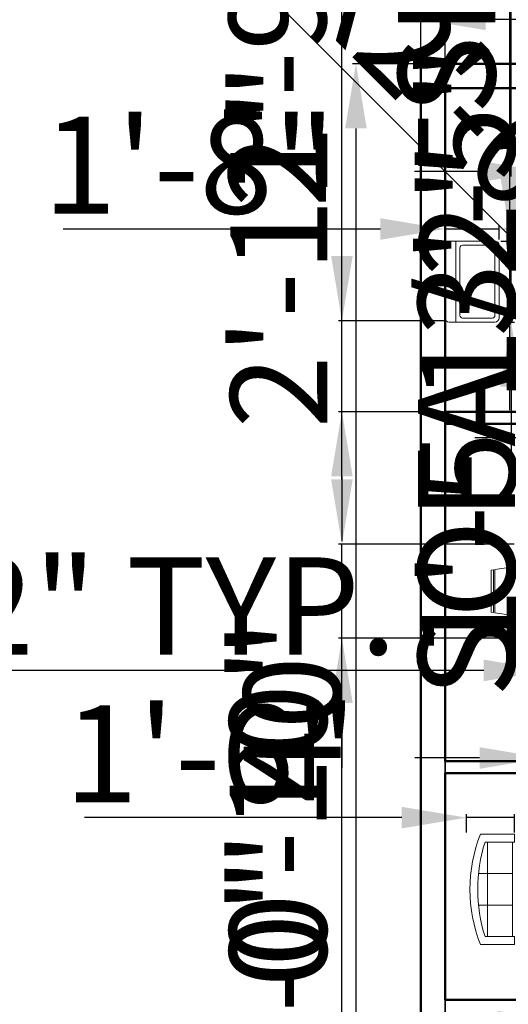
# Model space of a CAD drawing. Units: inches. Extents: x 1102 to 2414, y 295 to 1561.
# Tile 4 of 11: x 1429 to 1610, y 768 to 1133. Entities that reach past the tile are written whole.
import ezdxf

# ---------------------------------------------------------------- set-up
doc = ezdxf.new("R2010")
doc.units = ezdxf.units.IN
for name, color, linetype, lineweight in [('A-ANNO-DIMS', 2, 'Continuous', 18), ('A-FLOR-FIXT', 9, 'Continuous', 18), ('A-FURN', 8, 'Continuous', 18), ('A-WALL', 7, 'Continuous', 50)]:
    doc.layers.add(name, color=color, linetype=linetype, lineweight=lineweight)
doc.styles.get("Standard").update_dxf_attribs({"font": 'arial.ttf'})
doc.dimstyles.new('ISO-25', dxfattribs={"dimtxt": 36, "dimasz": 24, "dimexe": 1.25, "dimexo": 0.625, "dimtad": 1, "dimlunit": 4, "dimtxsty": 'Standard', "dimcen": 2.5, "dimadec": 0, "dimazin": 0, "dimtfac": 1, "dimtmove": 0, "dimatfit": 3, "dimfxl": 1, "dimarcsym": 0})

# ---------------------------------------------------------------- blocks, each defined once
blk = doc.blocks.new('*D1')
at = {"layer": 'A-ANNO-DIMS', "color": 0, "lineweight": -2, "transparency": 16777216}
for p, q in [((1577.54, 1117.38), (1577.54, 1134.48)), ((1601.54, 1133.23), (1793.54, 1133.23)), ((1817.54, 1117.38), (1817.54, 1134.48))]:
    blk.add_line(p, q, dxfattribs=at)
at = {"layer": 'A-ANNO-DIMS', "color": 0, "transparency": 16777216}
for points in [[(1601.54, 1137.23), (1601.54, 1129.23), (1577.54, 1133.23)], [(1793.54, 1137.23), (1793.54, 1129.23), (1817.54, 1133.23)]]:
    blk.add_solid(points, dxfattribs=at)
at = {"layer": 'Defpoints', "color": 0, "transparency": 16777216}
for p in [(1817.54, 1133.23), (1577.54, 1116.76), (1817.54, 1116.76)]:
    blk.add_point(p, dxfattribs=at)
at = {"layer": 'A-ANNO-DIMS', "color": 0, "transparency": 16777216, "insert": (1697.54, 1152.24), "char_height": 36, "attachment_point": 5}
blk.add_mtext("20'", dxfattribs=at)
blk = doc.blocks.new('*D2')
at = {"layer": 'A-ANNO-DIMS', "color": 0, "lineweight": -2, "transparency": 16777216}
for p, q in [((1576.92, 1116.76), (1552.25, 1116.76)), ((1553.5, 1092.76), (1553.5, 660.76)), ((1576.92, 636.76), (1552.25, 636.76))]:
    blk.add_line(p, q, dxfattribs=at)
at = {"layer": 'A-ANNO-DIMS', "color": 0, "transparency": 16777216}
for points in [[(1549.5, 1092.76), (1557.5, 1092.76), (1553.5, 1116.76)], [(1549.5, 660.76), (1557.5, 660.76), (1553.5, 636.76)]]:
    blk.add_solid(points, dxfattribs=at)
at = {"layer": 'Defpoints', "color": 0, "transparency": 16777216}
for p in [(1577.54, 1116.76), (1553.5, 636.76), (1577.54, 636.76)]:
    blk.add_point(p, dxfattribs=at)
at = {"layer": 'A-ANNO-DIMS', "color": 0, "transparency": 16777216, "insert": (1534.49, 876.76), "char_height": 36, "attachment_point": 5, "rotation": 90}
blk.add_mtext("40'", dxfattribs=at)
blk = doc.blocks.new('Sink-single - 30 in top')
blk.add_line((-15, -3.999996), (15, -3.999996))
for points in [[(-13.5, 0), (13.5, 0)], [(-15, -18.499996), (-15, -1.5)], [(15, -1.5), (15, -18.499996)], [(-13.5, -17.499996), (-13.5, -6.499996)], [(-12.5, -5.499996), (12.5, -5.499996)], [(13.5, -6.499996), (13.5, -17.499996)], [(13.5, -19.999996), (-13.5, -19.999996)], [(12.5, -18.499996), (-12.5, -18.499996)]]:
    blk.add_lwpolyline(points)
for radius in [1, 0.5]:
    blk.add_circle((0, -11.999996), radius)
for centre, radius, start, end in [((-13.5, -1.5), 1.5, 90, 180), ((13.5, -1.5), 1.5, 0, 90), ((-12.5, -6.499996), 1, 90, 180), ((12.5, -6.499996), 1, 0, 90), ((-12.5, -17.499996), 1, 180, 270), ((12.5, -17.499996), 1, 270, 0), ((-13.5, -18.499996), 1.5, 180, 270), ((13.5, -18.499996), 1.5, 270, 0)]:
    blk.add_arc(centre, radius, start, end)
blk = doc.blocks.new('Sofa - Roundback 7 ft.')
for p, q in [((-12.00002, -32.4421), (-12.00003, -6.5971)), ((11.99997, -32.4421), (11.99998, -6.5971)), ((-36.000027, -34), (-36.000027, -11.4696)), ((-35.999844, -13.3819), (35.9998, -13.3819)), ((35.99998, -34), (35.99998, -11.4696)), ((-36.000027, -32.4421), (35.99998, -32.4421))]:
    blk.add_line(p, q)
for points in [[(-36.000027, -34), (-42.000027, -34), (-42.000027, -8)], [(41.99998, -8), (41.99998, -34), (35.99998, -34)]]:
    blk.add_lwpolyline(points)
for centre, radius, start, end in [((0, -114.25), 114.25, 68.43141, 111.5686), ((-0.00001, -127.1968), 121.1968, 72.72033, 107.2797)]:
    blk.add_arc(centre, radius, start, end)
blk = doc.blocks.new('CHAIR-DINING')
for p, q in [((1.21, 7.75), (0, 0)), ((1.21, 7.75), (17.16, 7.75)), ((1.44, 9.2), (1.29, 8.23)), ((17.08, 8.23), (1.29, 8.23)), ((1.44, 9.2), (16.93, 9.2)), ((17.08, 8.23), (16.93, 9.2)), ((18.37, 0), (17.16, 7.75))]:
    blk.add_line(p, q)
blk = doc.blocks.new('*D17')
at = {"layer": 'A-ANNO-DIMS', "color": 0, "lineweight": -2, "transparency": 16777216}
for p, q in [((1600.9, 891.85), (1102.3, 891.8)), ((1624.9, 893.98), (1624.9, 890.6)), ((1643.27, 891.85), (1624.9, 891.85)), ((1643.27, 893.98), (1643.27, 890.6)), ((1667.27, 891.85), (1691.27, 891.85))]:
    blk.add_line(p, q, dxfattribs=at)
at = {"layer": 'A-ANNO-DIMS', "color": 0, "transparency": 16777216}
for points in [[(1600.9, 895.85), (1600.9, 887.85), (1624.9, 891.85)], [(1667.27, 895.85), (1667.27, 887.85), (1643.27, 891.85)]]:
    blk.add_solid(points, dxfattribs=at)
at = {"layer": 'Defpoints', "color": 0, "transparency": 16777216}
for p in [(1624.9, 894.6), (1643.27, 894.6), (1624.9, 891.85)]:
    blk.add_point(p, dxfattribs=at)
at = {"layer": 'A-ANNO-DIMS', "color": 0, "transparency": 16777216, "insert": (1339.6, 911.06), "char_height": 36, "attachment_point": 5, "rotation": 0.0057}
blk.add_mtext('CHAIR 1\'-6 1/2" TYP.', dxfattribs=at)
blk = doc.blocks.new('*D27')
at = {"layer": 'A-ANNO-DIMS', "color": 0, "lineweight": -2, "transparency": 16777216}
for p, q in [((1683.72, 1041.76), (1683.72, 1561.36)), ((1679.17, 1017.76), (1684.97, 1017.76)), ((1683.72, 983.26), (1683.72, 1017.76)), ((1679.17, 983.26), (1684.97, 983.26)), ((1683.72, 959.26), (1683.72, 935.26))]:
    blk.add_line(p, q, dxfattribs=at)
at = {"layer": 'A-ANNO-DIMS', "color": 0, "transparency": 16777216}
for points in [[(1679.72, 1041.76), (1687.72, 1041.76), (1683.72, 1017.76)], [(1679.72, 959.26), (1687.72, 959.26), (1683.72, 983.26)]]:
    blk.add_solid(points, dxfattribs=at)
at = {"layer": 'Defpoints', "color": 0, "transparency": 16777216}
for p in [(1678.54, 1017.76), (1683.72, 1017.76), (1678.54, 983.26)]:
    blk.add_point(p, dxfattribs=at)
at = {"layer": 'A-ANNO-DIMS', "color": 0, "transparency": 16777216, "insert": (1664.47, 1313.56), "char_height": 36, "attachment_point": 5, "rotation": 90}
blk.add_mtext('DOOR 2\'-10 1/2" TYP.', dxfattribs=at)
blk = doc.blocks.new('*D28')
at = {"layer": 'A-ANNO-DIMS', "color": 0, "lineweight": -2, "transparency": 16777216}
for p, q in [((1645.54, 982.63), (1645.54, 976.83)), ((1678.54, 982.63), (1678.54, 976.83)), ((1621.54, 978.08), (1597.54, 978.08)), ((1645.54, 978.08), (1678.54, 978.08)), ((1702.54, 978.08), (1947.85, 978.08))]:
    blk.add_line(p, q, dxfattribs=at)
at = {"layer": 'A-ANNO-DIMS', "color": 0, "transparency": 16777216}
for points in [[(1621.54, 982.08), (1621.54, 974.08), (1645.54, 978.08)], [(1702.54, 982.08), (1702.54, 974.08), (1678.54, 978.08)]]:
    blk.add_solid(points, dxfattribs=at)
at = {"layer": 'Defpoints', "color": 0, "transparency": 16777216}
for p in [(1645.54, 983.26), (1678.54, 983.26), (1678.54, 978.08)]:
    blk.add_point(p, dxfattribs=at)
at = {"layer": 'A-ANNO-DIMS', "color": 0, "transparency": 16777216, "insert": (1837.19, 997.09), "char_height": 36, "attachment_point": 5}
blk.add_mtext('2\'-9" TYP.', dxfattribs=at)
blk = doc.blocks.new('*D31')
at = {"layer": 'A-ANNO-DIMS', "color": 0, "lineweight": -2, "transparency": 16777216}
for p, q in [((1629.86, 764.63), (1629.86, 760.41)), ((1653.86, 764.63), (1653.86, 760.41)), ((1605.86, 761.66), (1581.86, 761.66)), ((1629.86, 761.66), (1653.86, 761.66)), ((1677.86, 761.66), (2225.36, 761.66))]:
    blk.add_line(p, q, dxfattribs=at)
at = {"layer": 'A-ANNO-DIMS', "color": 0, "transparency": 16777216}
for points in [[(1605.86, 765.66), (1605.86, 757.66), (1629.86, 761.66)], [(1677.86, 765.66), (1677.86, 757.66), (1653.86, 761.66)]]:
    blk.add_solid(points, dxfattribs=at)
at = {"layer": 'Defpoints', "color": 0, "transparency": 16777216}
for p in [(1629.86, 765.26), (1653.86, 765.26), (1653.86, 761.66)]:
    blk.add_point(p, dxfattribs=at)
at = {"layer": 'A-ANNO-DIMS', "color": 0, "transparency": 16777216, "insert": (1963.61, 780.91), "char_height": 36, "attachment_point": 5}
blk.add_mtext('DOOR LEAF 2\'-0" TYP.', dxfattribs=at)
blk = doc.blocks.new('*D32')
at = {"layer": 'A-ANNO-DIMS', "color": 0, "lineweight": -2, "transparency": 16777216}
for p, q in [((1657.46, 811.76), (1657.46, 1164.91)), ((1654.49, 787.76), (1658.71, 787.76)), ((1657.46, 765.26), (1657.46, 787.76)), ((1654.49, 765.26), (1658.71, 765.26)), ((1657.46, 741.26), (1657.46, 717.26))]:
    blk.add_line(p, q, dxfattribs=at)
at = {"layer": 'A-ANNO-DIMS', "color": 0, "transparency": 16777216}
for points in [[(1653.46, 811.76), (1661.46, 811.76), (1657.46, 787.76)], [(1653.46, 741.26), (1661.46, 741.26), (1657.46, 765.26)]]:
    blk.add_solid(points, dxfattribs=at)
at = {"layer": 'Defpoints', "color": 0, "transparency": 16777216}
for p in [(1653.86, 787.76), (1657.46, 787.76), (1653.86, 765.26)]:
    blk.add_point(p, dxfattribs=at)
at = {"layer": 'A-ANNO-DIMS', "color": 0, "transparency": 16777216, "insert": (1638.22, 1000.34), "char_height": 36, "attachment_point": 5, "rotation": 90}
blk.add_mtext('1\'-10 1/2" TYP.', dxfattribs=at)
blk = doc.blocks.new('*D33')
at = {"layer": 'A-ANNO-DIMS', "color": 0, "lineweight": -2, "transparency": 16777216}
for p, q in [((1623.16, 1080.7), (1623.16, 1075.57)), ((1653.16, 1080.7), (1653.16, 1075.57)), ((1599.16, 1076.82), (1575.16, 1076.82)), ((1623.16, 1076.82), (1653.16, 1076.82)), ((1677.16, 1076.82), (1989.06, 1076.82))]:
    blk.add_line(p, q, dxfattribs=at)
at = {"layer": 'A-ANNO-DIMS', "color": 0, "transparency": 16777216}
for points in [[(1599.16, 1080.82), (1599.16, 1072.82), (1623.16, 1076.82)], [(1677.16, 1080.82), (1677.16, 1072.82), (1653.16, 1076.82)]]:
    blk.add_solid(points, dxfattribs=at)
at = {"layer": 'Defpoints', "color": 0, "transparency": 16777216}
for p in [(1623.16, 1081.32), (1653.16, 1081.32), (1653.16, 1076.82)]:
    blk.add_point(p, dxfattribs=at)
at = {"layer": 'A-ANNO-DIMS', "color": 0, "transparency": 16777216, "insert": (1845.11, 1096.06), "char_height": 36, "attachment_point": 5}
blk.add_mtext('RANGE 2\'-6"', dxfattribs=at)
blk = doc.blocks.new('*D35')
at = {"layer": 'A-ANNO-DIMS', "color": 0, "lineweight": -2, "transparency": 16777216}
for p, q in [((1611.04, 1074.99), (1611.04, 1327.12)), ((1607.17, 1050.99), (1612.29, 1050.99)), ((1611.04, 1020.99), (1611.04, 1050.99)), ((1607.17, 1020.99), (1612.29, 1020.99)), ((1611.04, 996.99), (1611.04, 972.99))]:
    blk.add_line(p, q, dxfattribs=at)
at = {"layer": 'A-ANNO-DIMS', "color": 0, "transparency": 16777216}
for points in [[(1607.04, 1074.99), (1615.04, 1074.99), (1611.04, 1050.99)], [(1607.04, 996.99), (1615.04, 996.99), (1611.04, 1020.99)]]:
    blk.add_solid(points, dxfattribs=at)
at = {"layer": 'Defpoints', "color": 0, "transparency": 16777216}
for p in [(1606.54, 1050.99), (1611.04, 1050.99), (1606.54, 1020.99)]:
    blk.add_point(p, dxfattribs=at)
at = {"layer": 'A-ANNO-DIMS', "color": 0, "transparency": 16777216, "insert": (1591.81, 1213.06), "char_height": 36, "attachment_point": 5, "rotation": 90}
blk.add_mtext('SINK 2\'-6"', dxfattribs=at)
blk = doc.blocks.new('*D36')
at = {"layer": 'A-ANNO-DIMS', "color": 0, "lineweight": -2, "transparency": 16777216}
for p, q in [((1562.54, 1055.49), (1444.99, 1055.49)), ((1586.54, 1051.62), (1586.54, 1056.74)), ((1606.54, 1055.49), (1586.54, 1055.49)), ((1606.54, 1051.62), (1606.54, 1056.74)), ((1630.54, 1055.49), (1654.54, 1055.49))]:
    blk.add_line(p, q, dxfattribs=at)
at = {"layer": 'A-ANNO-DIMS', "color": 0, "transparency": 16777216}
for points in [[(1562.54, 1059.49), (1562.54, 1051.49), (1586.54, 1055.49)], [(1630.54, 1059.49), (1630.54, 1051.49), (1606.54, 1055.49)]]:
    blk.add_solid(points, dxfattribs=at)
at = {"layer": 'Defpoints', "color": 0, "transparency": 16777216}
for p in [(1586.54, 1055.49), (1586.54, 1050.99), (1606.54, 1050.99)]:
    blk.add_point(p, dxfattribs=at)
at = {"layer": 'A-ANNO-DIMS', "color": 0, "transparency": 16777216, "insert": (1491.76, 1074.5), "char_height": 36, "attachment_point": 5}
blk.add_mtext('1\'-8"', dxfattribs=at)
blk = doc.blocks.new('*D37')
at = {"layer": 'A-ANNO-DIMS', "color": 0, "lineweight": -2, "transparency": 16777216}
for p, q in [((1618.46, 855.15), (1618.46, 1126.82)), ((1612.94, 831.15), (1619.71, 831.15)), ((1618.46, 790.23), (1618.46, 831.15)), ((1612.94, 790.23), (1619.71, 790.23)), ((1618.46, 766.23), (1618.46, 742.23))]:
    blk.add_line(p, q, dxfattribs=at)
at = {"layer": 'A-ANNO-DIMS', "color": 0, "transparency": 16777216}
for points in [[(1614.46, 855.15), (1622.46, 855.15), (1618.46, 831.15)], [(1614.46, 766.23), (1622.46, 766.23), (1618.46, 790.23)]]:
    blk.add_solid(points, dxfattribs=at)
at = {"layer": 'Defpoints', "color": 0, "transparency": 16777216}
for p in [(1612.32, 831.15), (1618.46, 831.15), (1612.32, 790.23)]:
    blk.add_point(p, dxfattribs=at)
at = {"layer": 'A-ANNO-DIMS', "color": 0, "transparency": 16777216, "insert": (1599.19, 1002.98), "char_height": 36, "attachment_point": 5, "rotation": 90}
blk.add_mtext('SOFA 3\'-5"', dxfattribs=at)
blk = doc.blocks.new('*D38')
at = {"layer": 'A-ANNO-DIMS', "color": 0, "lineweight": -2, "transparency": 16777216}
for p, q in [((1570.46, 837.28), (1452.9, 837.28)), ((1594.46, 831.77), (1594.46, 838.53)), ((1612.32, 837.28), (1594.46, 837.28)), ((1612.32, 831.77), (1612.32, 838.53)), ((1636.32, 837.28), (1660.32, 837.28))]:
    blk.add_line(p, q, dxfattribs=at)
at = {"layer": 'A-ANNO-DIMS', "color": 0, "transparency": 16777216}
for points in [[(1570.46, 841.28), (1570.46, 833.28), (1594.46, 837.28)], [(1636.32, 841.28), (1636.32, 833.28), (1612.32, 837.28)]]:
    blk.add_solid(points, dxfattribs=at)
at = {"layer": 'Defpoints', "color": 0, "transparency": 16777216}
for p in [(1594.46, 837.28), (1594.46, 831.15), (1612.32, 831.15)]:
    blk.add_point(p, dxfattribs=at)
at = {"layer": 'A-ANNO-DIMS', "color": 0, "transparency": 16777216, "insert": (1499.68, 856.29), "char_height": 36, "attachment_point": 5}
blk.add_mtext('1\'-6"', dxfattribs=at)
blk = doc.blocks.new('*D39')
at = {"layer": 'A-ANNO-DIMS', "color": 0, "lineweight": -2, "transparency": 16777216}
for p, q in [((1599.32, 859.39), (1575.32, 859.39)), ((1623.32, 855.67), (1623.32, 860.64)), ((1623.32, 859.39), (1652.27, 859.39)), ((1652.27, 855.67), (1652.27, 860.64)), ((1676.27, 859.39), (2075.12, 859.39))]:
    blk.add_line(p, q, dxfattribs=at)
at = {"layer": 'A-ANNO-DIMS', "color": 0, "transparency": 16777216}
for points in [[(1599.32, 863.39), (1599.32, 855.39), (1623.32, 859.39)], [(1676.27, 863.39), (1676.27, 855.39), (1652.27, 859.39)]]:
    blk.add_solid(points, dxfattribs=at)
at = {"layer": 'Defpoints', "color": 0, "transparency": 16777216}
for p in [(1652.27, 859.39), (1623.32, 855.05), (1652.27, 855.05)]:
    blk.add_point(p, dxfattribs=at)
at = {"layer": 'A-ANNO-DIMS', "color": 0, "transparency": 16777216, "insert": (1887.69, 878.64), "char_height": 36, "attachment_point": 5}
blk.add_mtext('LOVESEAT 2\'-5"', dxfattribs=at)
blk = doc.blocks.new('*D40')
at = {"layer": 'A-ANNO-DIMS', "color": 0, "lineweight": -2, "transparency": 16777216}
for p, q in [((1618.98, 879.05), (1618.98, 1080.49)), ((1622.7, 855.05), (1617.73, 855.05)), ((1618.98, 837.36), (1618.98, 855.05)), ((1622.7, 837.36), (1617.73, 837.36)), ((1618.98, 813.36), (1618.98, 789.36))]:
    blk.add_line(p, q, dxfattribs=at)
at = {"layer": 'A-ANNO-DIMS', "color": 0, "transparency": 16777216}
for points in [[(1614.98, 879.05), (1622.98, 879.05), (1618.98, 855.05)], [(1614.98, 813.36), (1622.98, 813.36), (1618.98, 837.36)]]:
    blk.add_solid(points, dxfattribs=at)
at = {"layer": 'Defpoints', "color": 0, "transparency": 16777216}
for p in [(1618.98, 855.05), (1623.32, 855.05), (1623.32, 837.36)]:
    blk.add_point(p, dxfattribs=at)
at = {"layer": 'A-ANNO-DIMS', "color": 0, "transparency": 16777216, "insert": (1599.74, 991.77), "char_height": 36, "attachment_point": 5, "rotation": 90}
blk.add_mtext('1\'-5 1/2"', dxfattribs=at)
blk = doc.blocks.new('*D46')
at = {"layer": 'A-ANNO-DIMS', "color": 0, "lineweight": -2, "transparency": 16777216}
for p, q in [((1732.04, 857.63), (1732.04, 606.26)), ((1586.54, 853.13), (1586.54, 606.26)), ((1610.54, 607.51), (1708.04, 607.51)), ((1732.04, 607.51), (1961.46, 607.51))]:
    blk.add_line(p, q, dxfattribs=at)
at = {"layer": 'A-ANNO-DIMS', "color": 0, "transparency": 16777216}
for points in [[(1610.54, 611.51), (1610.54, 603.51), (1586.54, 607.51)], [(1708.04, 611.51), (1708.04, 603.51), (1732.04, 607.51)]]:
    blk.add_solid(points, dxfattribs=at)
at = {"layer": 'Defpoints', "color": 0, "transparency": 16777216}
for p in [(1732.04, 858.26), (1586.54, 853.76), (1732.04, 607.51)]:
    blk.add_point(p, dxfattribs=at)
at = {"layer": 'A-ANNO-DIMS', "color": 0, "transparency": 16777216, "insert": (1858.75, 626.75), "char_height": 36, "attachment_point": 5}
blk.add_mtext('12\'-1 1/2"', dxfattribs=at)
blk = doc.blocks.new('*D50')
at = {"layer": 'A-ANNO-DIMS', "color": 0, "lineweight": -2, "transparency": 16777216}
for p, q in [((1586.54, 987.13), (1586.54, 606.26)), ((1654.54, 987.13), (1654.54, 606.26)), ((1610.54, 607.51), (1630.54, 607.51)), ((1654.54, 607.51), (1775.49, 607.51))]:
    blk.add_line(p, q, dxfattribs=at)
at = {"layer": 'A-ANNO-DIMS', "color": 0, "transparency": 16777216}
for points in [[(1610.54, 611.51), (1610.54, 603.51), (1586.54, 607.51)], [(1630.54, 611.51), (1630.54, 603.51), (1654.54, 607.51)]]:
    blk.add_solid(points, dxfattribs=at)
at = {"layer": 'Defpoints', "color": 0, "transparency": 16777216}
for p in [(1586.54, 987.76), (1654.54, 987.76), (1654.54, 607.51)]:
    blk.add_point(p, dxfattribs=at)
at = {"layer": 'A-ANNO-DIMS', "color": 0, "transparency": 16777216, "insert": (1727.02, 626.52), "char_height": 36, "attachment_point": 5}
blk.add_mtext('5\'-8"', dxfattribs=at)
blk = doc.blocks.new('*D53')
at = {"layer": 'A-ANNO-DIMS', "color": 0, "lineweight": -2, "transparency": 16777216}
for p, q in [((1586.54, 988.38), (1586.54, 1147.26)), ((1610.54, 988.38), (1610.54, 1147.26)), ((1562.54, 1146.01), (1538.54, 1146.01)), ((1586.54, 1146.01), (1610.54, 1146.01)), ((1634.54, 1146.01), (1756.11, 1146.01))]:
    blk.add_line(p, q, dxfattribs=at)
at = {"layer": 'A-ANNO-DIMS', "color": 0, "transparency": 16777216}
for points in [[(1562.54, 1150.01), (1562.54, 1142.01), (1586.54, 1146.01)], [(1634.54, 1150.01), (1634.54, 1142.01), (1610.54, 1146.01)]]:
    blk.add_solid(points, dxfattribs=at)
at = {"layer": 'Defpoints', "color": 0, "transparency": 16777216}
for p in [(1610.54, 1146.01), (1586.54, 987.76), (1610.54, 987.76)]:
    blk.add_point(p, dxfattribs=at)
at = {"layer": 'A-ANNO-DIMS', "color": 0, "transparency": 16777216, "insert": (1707.32, 1165.02), "char_height": 36, "attachment_point": 5}
blk.add_mtext('2\'-0"', dxfattribs=at)
blk = doc.blocks.new('*D55')
at = {"layer": 'A-ANNO-DIMS', "color": 0, "lineweight": -2, "transparency": 16777216}
for p, q in [((1586.54, 722.38), (1586.54, 1147.26)), ((1622.54, 722.38), (1622.54, 1147.26)), ((1562.54, 1146.01), (1538.54, 1146.01)), ((1586.54, 1146.01), (1622.54, 1146.01)), ((1646.54, 1146.01), (1767.47, 1146.01))]:
    blk.add_line(p, q, dxfattribs=at)
at = {"layer": 'A-ANNO-DIMS', "color": 0, "transparency": 16777216}
for points in [[(1562.54, 1150.01), (1562.54, 1142.01), (1586.54, 1146.01)], [(1646.54, 1150.01), (1646.54, 1142.01), (1622.54, 1146.01)]]:
    blk.add_solid(points, dxfattribs=at)
at = {"layer": 'Defpoints', "color": 0, "transparency": 16777216}
for p in [(1622.54, 1146.01), (1586.54, 721.76), (1622.54, 721.76)]:
    blk.add_point(p, dxfattribs=at)
at = {"layer": 'A-ANNO-DIMS', "color": 0, "transparency": 16777216, "insert": (1719.01, 1165.03), "char_height": 36, "attachment_point": 5}
blk.add_mtext('3\'-0"', dxfattribs=at)
blk = doc.blocks.new('*D56')
at = {"layer": 'A-ANNO-DIMS', "color": 0, "lineweight": -2, "transparency": 16777216}
for p, q in [((1548.29, 705.76), (1548.29, 826.68)), ((1585.92, 681.76), (1547.04, 681.76)), ((1548.29, 645.76), (1548.29, 681.76)), ((1585.92, 645.76), (1547.04, 645.76)), ((1548.29, 621.76), (1548.29, 597.76))]:
    blk.add_line(p, q, dxfattribs=at)
at = {"layer": 'A-ANNO-DIMS', "color": 0, "transparency": 16777216}
for points in [[(1544.29, 705.76), (1552.29, 705.76), (1548.29, 681.76)], [(1544.29, 621.76), (1552.29, 621.76), (1548.29, 645.76)]]:
    blk.add_solid(points, dxfattribs=at)
at = {"layer": 'Defpoints', "color": 0, "transparency": 16777216}
for p in [(1548.29, 681.76), (1586.54, 681.76), (1586.54, 645.76)]:
    blk.add_point(p, dxfattribs=at)
at = {"layer": 'A-ANNO-DIMS', "color": 0, "transparency": 16777216, "insert": (1529.28, 778.22), "char_height": 36, "attachment_point": 5, "rotation": 90}
blk.add_mtext('3\'-0"', dxfattribs=at)
blk = doc.blocks.new('*D57')
at = {"layer": 'A-ANNO-DIMS', "color": 0, "lineweight": -2, "transparency": 16777216}
for p, q in [((1548.29, 755.76), (1548.29, 904.68)), ((1585.92, 731.76), (1547.04, 731.76)), ((1548.29, 721.76), (1548.29, 731.76)), ((1585.92, 721.76), (1547.04, 721.76)), ((1548.29, 697.76), (1548.29, 673.76))]:
    blk.add_line(p, q, dxfattribs=at)
at = {"layer": 'A-ANNO-DIMS', "color": 0, "transparency": 16777216}
for points in [[(1544.29, 755.76), (1552.29, 755.76), (1548.29, 731.76)], [(1544.29, 697.76), (1552.29, 697.76), (1548.29, 721.76)]]:
    blk.add_solid(points, dxfattribs=at)
at = {"layer": 'Defpoints', "color": 0, "transparency": 16777216}
for p in [(1548.29, 731.76), (1586.54, 731.76), (1586.54, 721.76)]:
    blk.add_point(p, dxfattribs=at)
at = {"layer": 'A-ANNO-DIMS', "color": 0, "transparency": 16777216, "insert": (1529.29, 842.22), "char_height": 36, "attachment_point": 5, "rotation": 90}
blk.add_mtext('0\'-10"', dxfattribs=at)
blk = doc.blocks.new('*D59')
at = {"layer": 'A-ANNO-DIMS', "color": 0, "lineweight": -2, "transparency": 16777216}
for p, q in [((1548.29, 962.66), (1548.29, 1112.19)), ((1612.15, 938.66), (1547.04, 938.66)), ((1548.29, 903.8), (1548.29, 938.66)), ((1612.15, 903.8), (1547.04, 903.8)), ((1548.29, 879.8), (1548.29, 855.8))]:
    blk.add_line(p, q, dxfattribs=at)
at = {"layer": 'A-ANNO-DIMS', "color": 0, "transparency": 16777216}
for points in [[(1544.29, 962.66), (1552.29, 962.66), (1548.29, 938.66)], [(1544.29, 879.8), (1552.29, 879.8), (1548.29, 903.8)]]:
    blk.add_solid(points, dxfattribs=at)
at = {"layer": 'Defpoints', "color": 0, "transparency": 16777216}
for p in [(1548.29, 938.66), (1612.78, 938.66), (1612.78, 903.8)]:
    blk.add_point(p, dxfattribs=at)
at = {"layer": 'A-ANNO-DIMS', "color": 0, "transparency": 16777216, "insert": (1529.6, 1049.43), "char_height": 36, "attachment_point": 5, "rotation": 90}
blk.add_mtext('2\'-11"', dxfattribs=at)
blk = doc.blocks.new('*D60')
at = {"layer": 'A-ANNO-DIMS', "color": 0, "lineweight": -2, "transparency": 16777216}
for p, q in [((1586.54, 1108.38), (1586.54, 1147.26)), ((1623.16, 1107.95), (1623.16, 1147.26)), ((1562.54, 1146.01), (1538.54, 1146.01)), ((1586.54, 1146.01), (1623.16, 1146.01)), ((1647.16, 1146.01), (1851.97, 1146.01))]:
    blk.add_line(p, q, dxfattribs=at)
at = {"layer": 'A-ANNO-DIMS', "color": 0, "transparency": 16777216}
for points in [[(1562.54, 1150.01), (1562.54, 1142.01), (1586.54, 1146.01)], [(1647.16, 1150.01), (1647.16, 1142.01), (1623.16, 1146.01)]]:
    blk.add_solid(points, dxfattribs=at)
at = {"layer": 'Defpoints', "color": 0, "transparency": 16777216}
for p in [(1623.16, 1146.01), (1586.54, 1107.76), (1623.16, 1107.32)]:
    blk.add_point(p, dxfattribs=at)
at = {"layer": 'A-ANNO-DIMS', "color": 0, "transparency": 16777216, "insert": (1761.57, 1165.26), "char_height": 36, "attachment_point": 5}
blk.add_mtext('3\'-0 1/2"', dxfattribs=at)
blk = doc.blocks.new('*D61')
at = {"layer": 'A-ANNO-DIMS', "color": 0, "lineweight": -2, "transparency": 16777216}
for p, q in [((1548.29, 1045.43), (1548.29, 1250.88)), ((1586.36, 1021.43), (1547.04, 1021.43)), ((1548.29, 987.76), (1548.29, 1021.43)), ((1585.92, 987.76), (1547.04, 987.76)), ((1548.29, 963.76), (1548.29, 939.76))]:
    blk.add_line(p, q, dxfattribs=at)
at = {"layer": 'A-ANNO-DIMS', "color": 0, "transparency": 16777216}
for points in [[(1544.29, 1045.43), (1552.29, 1045.43), (1548.29, 1021.43)], [(1544.29, 963.76), (1552.29, 963.76), (1548.29, 987.76)]]:
    blk.add_solid(points, dxfattribs=at)
at = {"layer": 'Defpoints', "color": 0, "transparency": 16777216}
for p in [(1548.29, 1021.43), (1586.98, 1021.43), (1586.54, 987.76)]:
    blk.add_point(p, dxfattribs=at)
at = {"layer": 'A-ANNO-DIMS', "color": 0, "transparency": 16777216, "insert": (1529.06, 1160.15), "char_height": 36, "attachment_point": 5, "rotation": 90}
blk.add_mtext('2\'-9 1/2"', dxfattribs=at)
blk = doc.blocks.new('*D63')
at = {"layer": 'A-ANNO-DIMS', "color": 0, "lineweight": -2, "transparency": 16777216}
for p, q in [((1654.54, 982.63), (1654.54, 606.26)), ((1678.54, 982.63), (1678.54, 606.26)), ((1630.54, 607.51), (1606.54, 607.51)), ((1654.54, 607.51), (1678.54, 607.51)), ((1702.54, 607.51), (1824.11, 607.51))]:
    blk.add_line(p, q, dxfattribs=at)
at = {"layer": 'A-ANNO-DIMS', "color": 0, "transparency": 16777216}
for points in [[(1630.54, 611.51), (1630.54, 603.51), (1654.54, 607.51)], [(1702.54, 611.51), (1702.54, 603.51), (1678.54, 607.51)]]:
    blk.add_solid(points, dxfattribs=at)
at = {"layer": 'Defpoints', "color": 0, "transparency": 16777216}
for p in [(1654.54, 983.26), (1678.54, 983.26), (1678.54, 607.51)]:
    blk.add_point(p, dxfattribs=at)
at = {"layer": 'A-ANNO-DIMS', "color": 0, "transparency": 16777216, "insert": (1775.32, 626.52), "char_height": 36, "attachment_point": 5}
blk.add_mtext('2\'-0"', dxfattribs=at)
blk = doc.blocks.new('*D68')
at = {"layer": 'A-ANNO-DIMS', "color": 0, "lineweight": -2, "transparency": 16777216}
for p, q in [((1527.48, 1135.83), (1637.36, 1025.94)), ((1675.54, 987.76), (1654.33, 1008.97))]:
    blk.add_line(p, q, dxfattribs=at)
at = {"layer": 'A-ANNO-DIMS', "color": 0, "transparency": 16777216}
blk.add_solid([(1640.19, 1028.77), (1634.53, 1023.12), (1654.33, 1008.97)], dxfattribs=at)
at = {"layer": 'Defpoints', "color": 0, "transparency": 16777216}
for p in [(1654.33, 1008.97), (1675.54, 987.76)]:
    blk.add_point(p, dxfattribs=at)
at = {"layer": 'A-ANNO-DIMS', "color": 0, "transparency": 16777216, "insert": (1587.37, 1102.81), "char_height": 36, "attachment_point": 5, "rotation": 314.9996}
blk.add_mtext('R2\'-6"', dxfattribs=at)

msp = doc.modelspace()

# ---------------------------------------------------------------- linework, layer by layer
at = {"layer": 'A-WALL'}
for p, q in [((1817.544, 1116.76), (1577.544, 1116.76)), ((1577.544, 1116.76), (1577.544, 636.76)), ((1586.544, 1107.76), (1586.544, 858.26)), ((1684.544, 1107.76), (1586.544, 1107.76)), ((1654.544, 987.76), (1586.544, 987.76)), ((1654.544, 983.26), (1586.544, 983.26)), ((1684.544, 858.26), (1586.544, 858.26)), ((1689.044, 853.76), (1586.544, 853.76)), ((1586.544, 853.76), (1586.544, 769.76)), ((1632.864, 769.76), (1586.544, 769.76))]:
    msp.add_line(p, q, dxfattribs=at)

# ---------------------------------------------------------------- block references
at = {"layer": 'A-FLOR-FIXT', "rotation": 90}
msp.add_blockref('Sink-single - 30 in top', (1586.544, 1035.991), dxfattribs=at)
at = {"layer": 'A-FURN', "rotation": 90.00584970642711}
msp.add_blockref('CHAIR-DINING', (1612.782, 912.048), dxfattribs=at)
at = {"layer": 'A-FURN', "xscale": 0.4870553998389214, "yscale": 0.4870553998389214, "zscale": 0.4870553998389214, "rotation": 90}
msp.add_blockref('Sofa - Roundback 7 ft.', (1595.759, 810.689), dxfattribs=at)

# ---------------------------------------------------------------- dimensions: what is measured, and where the dimension line sits
at = {"layer": 'A-ANNO-DIMS'}
for base, p1, p2, angle, text, picture, middle in [((1683.719, 1017.76), (1678.544, 983.26), (1678.544, 1017.76), 90, 'DOOR <> TYP.', '*D27', (1664.468, 1313.559)), ((1611.044, 1050.991), (1606.544, 1020.991), (1606.544, 1050.991), 90, 'SINK <>', '*D35', (1591.805, 1213.055)), ((1657.464, 787.76), (1653.864, 765.26), (1653.864, 787.76), 90, '<> TYP.', '*D32', (1638.225, 1000.337)), ((1618.456, 831.145), (1612.319, 790.233), (1612.319, 831.145), 90, 'SOFA <>', '*D37', (1599.192, 1002.983)), ((1624.9, 891.848), (1643.269, 894.605), (1624.9, 894.603), 180.00567, 'CHAIR <> TYP.', '*D17', (1339.596, 911.058))]:
    dim = msp.add_linear_dim(base=base, p1=p1, p2=p2, angle=angle, text=text, dimstyle='ISO-25', override={"dimdec": 1, "dimlfac": 1, "dimrnd": 0, "dimzin": 1, "dimdsep": 46, "dimlunit": 4, "dimfrac": 2}, dxfattribs=at)
    dim.commit()
    dim.dimension.update_dxf_attribs({"geometry": picture, "text_midpoint": middle})
for base, p1, p2, angle, override, picture, middle in [((1548.294, 1021.43), (1586.544, 987.76), (1586.983, 1021.43), 90, {"dimdec": 1, "dimlfac": 1, "dimrnd": 0, "dimzin": 1, "dimdsep": 46, "dimlunit": 4, "dimfrac": 2}, '*D61', (1529.055, 1160.153)), ((1548.294, 938.663), (1612.778, 903.803), (1612.778, 938.663), 90, {"dimdec": 1, "dimlfac": 1, "dimrnd": 0, "dimzin": 1, "dimdsep": 46, "dimlunit": 4, "dimfrac": 2}, '*D59', (1529.595, 1049.429)), ((1553.496, 636.76), (1577.544, 1116.76), (1577.544, 636.76), 90, {"dimclrd": 0, "dimclre": 0, "dimclrt": 0}, '*D2', (1534.49, 876.76)), ((1586.544, 1055.491), (1606.544, 1050.991), (1586.544, 1050.991), 180, {"dimdec": 1, "dimlfac": 1, "dimrnd": 0, "dimzin": 1, "dimdsep": 46, "dimlunit": 4, "dimfrac": 2}, '*D36', (1491.765, 1074.497)), ((1618.978, 855.046), (1623.32, 837.356), (1623.32, 855.046), 90, {"dimdec": 1, "dimlfac": 1, "dimrnd": 0, "dimzin": 1, "dimdsep": 46, "dimlunit": 4, "dimfrac": 2}, '*D40', (1599.739, 991.768)), ((1548.294, 731.76), (1586.544, 721.76), (1586.544, 731.76), 90, {"dimdec": 1, "dimlfac": 1, "dimrnd": 0, "dimzin": 1, "dimdsep": 46, "dimlunit": 4, "dimfrac": 2}, '*D57', (1529.288, 842.218)), ((1594.46, 837.282), (1612.319, 831.145), (1594.46, 831.145), 180, {"dimdec": 1, "dimlfac": 1, "dimrnd": 0, "dimzin": 1, "dimdsep": 46, "dimlunit": 4, "dimfrac": 2}, '*D38', (1499.681, 856.288)), ((1548.294, 681.76), (1586.544, 645.76), (1586.544, 681.76), 90, {"dimdec": 1, "dimlfac": 1, "dimrnd": 0, "dimzin": 1, "dimdsep": 46, "dimlunit": 4, "dimfrac": 2}, '*D56', (1529.276, 778.221))]:
    dim = msp.add_linear_dim(base=base, p1=p1, p2=p2, angle=angle, dimstyle='ISO-25', override=override, dxfattribs=at)
    dim.commit()
    dim.dimension.update_dxf_attribs({"geometry": picture, "text_midpoint": middle})
for base, p1, p2, override, picture, middle in [((1623.162, 1146.01), (1586.544, 1107.76), (1623.162, 1107.321), {"dimdec": 1, "dimlfac": 1, "dimrnd": 0, "dimzin": 1, "dimdsep": 46, "dimlunit": 4, "dimfrac": 2}, '*D60', (1761.566, 1165.261)), ((1622.544, 1146.01), (1586.544, 721.76), (1622.544, 721.76), {"dimdec": 1, "dimlfac": 1, "dimrnd": 0, "dimzin": 1, "dimdsep": 46, "dimlunit": 4, "dimfrac": 2}, '*D55', (1719.005, 1165.028)), ((1610.544, 1146.01), (1586.544, 987.76), (1610.544, 987.76), {"dimdec": 1, "dimlfac": 1, "dimrnd": 0, "dimzin": 1, "dimdsep": 46, "dimlunit": 4, "dimfrac": 2}, '*D53', (1707.325, 1165.015)), ((1817.544, 1133.235), (1577.544, 1116.76), (1817.544, 1116.76), {"dimclrd": 0, "dimclre": 0, "dimclrt": 0}, '*D1', (1697.544, 1152.24)), ((1654.544, 607.51), (1586.544, 987.76), (1654.544, 987.76), {"dimdec": 1, "dimlfac": 1, "dimrnd": 0, "dimzin": 1, "dimdsep": 46, "dimlunit": 4, "dimfrac": 2}, '*D50', (1727.018, 626.515)), ((1678.544, 607.51), (1654.544, 983.26), (1678.544, 983.26), {"dimdec": 1, "dimlfac": 1, "dimrnd": 0, "dimzin": 1, "dimdsep": 46, "dimlunit": 4, "dimfrac": 2}, '*D63', (1775.325, 626.515)), ((1732.044, 607.51), (1586.544, 853.76), (1732.044, 858.26), {"dimdec": 1, "dimlfac": 1, "dimrnd": 0, "dimzin": 1, "dimdsep": 46, "dimlunit": 4, "dimfrac": 2}, '*D46', (1858.751, 626.749))]:
    dim = msp.add_linear_dim(base=base, p1=p1, p2=p2, dimstyle='ISO-25', override=override, dxfattribs=at)
    dim.commit()
    dim.dimension.update_dxf_attribs({"geometry": picture, "text_midpoint": middle})
dim = msp.add_radius_dim(center=(1675.544, 987.76), mpoint=(1654.331, 1008.973), dimstyle='ISO-25', override={"dimdec": 1, "dimlfac": 1, "dimrnd": 0, "dimzin": 1, "dimdsep": 46, "dimlunit": 4, "dimfrac": 2}, dxfattribs=at)
dim.commit()
dim.dimension.update_dxf_attribs({"geometry": '*D68', "text_midpoint": (1587.373, 1102.811)})
for base, p1, p2, text, picture, middle in [((1653.162, 1076.821), (1623.162, 1081.321), (1653.162, 1081.321), 'RANGE <>', '*D33', (1845.112, 1096.06)), ((1678.544, 978.085), (1645.544, 983.26), (1678.544, 983.26), '<> TYP.', '*D28', (1837.195, 997.09)), ((1652.268, 859.388), (1623.32, 855.046), (1652.268, 855.046), 'LOVESEAT <>', '*D39', (1887.695, 878.64)), ((1653.864, 761.66), (1629.864, 765.26), (1653.864, 765.26), 'DOOR LEAF <> TYP.', '*D31', (1963.611, 780.911))]:
    dim = msp.add_linear_dim(base=base, p1=p1, p2=p2, text=text, dimstyle='ISO-25', override={"dimdec": 1, "dimlfac": 1, "dimrnd": 0, "dimzin": 1, "dimdsep": 46, "dimlunit": 4, "dimfrac": 2}, dxfattribs=at)
    dim.commit()
    dim.dimension.update_dxf_attribs({"geometry": picture, "text_midpoint": middle})

doc.saveas('drawing.dxf')
